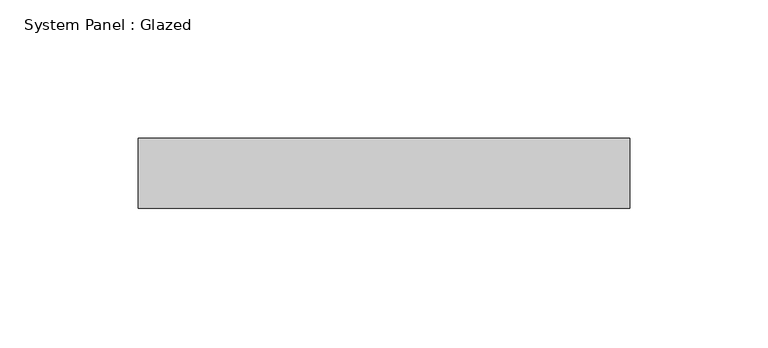
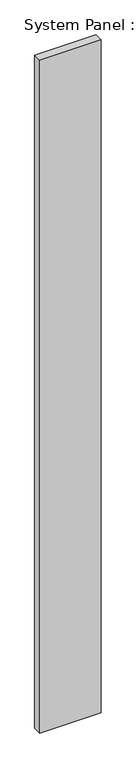
"""IFC4 building model written with IfcOpenShell, lengths in millimetres: plate geometry, System Panel : Glazed."""

from ifc_helpers import new_model, si_unit, origin, origin_with_axes, place, context, project, spatial, polyline, outline, extrude, source, transform, mapped, element, save


def system_panel_glazed_ebf67a72(model_context):
    return source(origin(), model_context, "Body", "SweptSolid", [
        extrude(outline(polyline([(88.9, 19.05), (-88.9, 19.05), (-88.9, 44.45), (88.9, 44.45), (88.9, 19.05)])), origin_with_axes(), (0.0, 0.0, 1.0), 2060.8644013),
    ])


if __name__ == "__main__":
    model = new_model("IFC4")
    model_context = context("Model", 3, world=origin())
    ifc_project = project(units=[si_unit("LENGTHUNIT", "METRE", prefix="MILLI")], contexts=[model_context])
    site = spatial("IfcSite", under=ifc_project)
    building = spatial("IfcBuilding", under=site)
    placement = place(None, origin())
    system_panel_glazed_shape = system_panel_glazed_ebf67a72(model_context)
    element("IfcPlate", 1, ObjectType="System Panel : Glazed", at=placement, inside=building, context=model_context, shape_type="MappedRepresentation", body=[
        mapped(system_panel_glazed_shape, transform((0.0, 0.0, 0.0), x_axis=(1.0, 0.0, 0.0), y_axis=(0.0, 1.0, 0.0), z_axis=(0.0, 0.0, 1.0))),
    ])
    save(model, "model.ifc")

# Revit data of these elements
# Type "System Panel : Glazed"
#   Construction Type Id = "GSP4R"
#   Analytic Construction = "1/8 in Pilkington single glazing"
#   Visual Light Transmittance = 0.9
#   Solar Heat Gain Coefficient = 0.86
#   Heat Transfer Coefficient (U) = 1.18115 BTU/(h·ft²·°F)
#   Define Thermal Properties by = 1
# Element 1 (IfcPlate, "System Panel : Glazed")
#   Materials on its faces: "Glass"
# Materials
#   "Glass": class "Glass", colour RGB 0 128 192, transparency 0.75, Description = "Soda Lime Glass", Cost = 0
